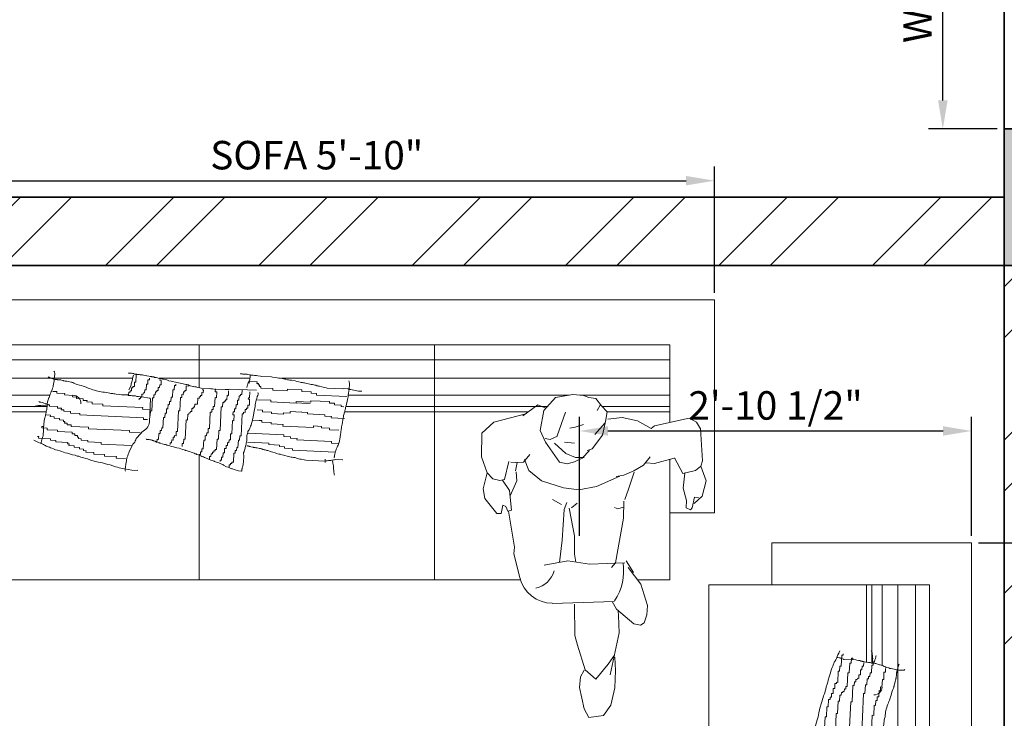
# Model space of a CAD drawing. Units: inches. Extents: x -138 to 270, y 8284 to 8764.
# Tile 8 of 10: x 112 to 198, y 8444 to 8506. Entities that reach past the tile are written whole.
import ezdxf

# ---------------------------------------------------------------- set-up
doc = ezdxf.new("R2010")
doc.units = ezdxf.units.IN
for name, color, linetype, lineweight in [('A-ANNO-DIMS', 2, 'Continuous', 18), ('FURNITURE', 8, 'Continuous', 15), ('FURNITURE1', 8, 'Continuous', 15), ('WALL', 8, 'Continuous', 35)]:
    doc.layers.add(name, color=color, linetype=linetype, lineweight=lineweight)
doc.layers.add('A-COLS', color=252, linetype='Continuous', lineweight=35, true_color=0x939598)
doc.layers.add('A-WALL-PATT', color=32, linetype='Continuous', lineweight=9, true_color=0xbc761a)
doc.styles.get("Standard").update_dxf_attribs({"font": 'arial.ttf'})
doc.dimstyles.new('ISO-25', dxfattribs={"dimtxt": 2.5, "dimasz": 2.5, "dimexe": 1.25, "dimexo": 0.625, "dimtad": 1, "dimdec": 0, "dimlunit": 3, "dimtxsty": 'Standard', "dimcen": 2.5, "dimadec": 0, "dimazin": 0, "dimtfac": 1, "dimtdec": 0, "dimtmove": 0, "dimatfit": 3, "dimfxl": 1, "dimarcsym": 0})

# ---------------------------------------------------------------- blocks, each defined once
blk = doc.blocks.new('A$C48A43CE3')
at = {"layer": 'FURNITURE1', "ltscale": 2}
for p, q in [((21.39, 35.19), (21.36, 35.19)), ((21.42, 35.15), (21.39, 35.19)), ((21.68, 35.14), (21.42, 35.15)), ((21.74, 34.36), (21.64, 34.07)), ((21.77, 35.11), (21.68, 35.14)), ((21.77, 34.49), (21.74, 34.36)), ((21.88, 35.1), (21.77, 35.11)), ((21.78, 34.59), (21.77, 34.49)), ((21.84, 34.84), (21.78, 34.59)), ((21.88, 34.94), (21.84, 34.84)), ((22, 35.06), (21.88, 35.1)), ((21.99, 34.24), (21.97, 33.79)), ((22.13, 34.23), (21.99, 34.24)), ((22.18, 35.06), (22, 35.06)), ((22.16, 34.99), (22.13, 34.23)), ((22.23, 35.02), (22.18, 35.06)), ((22.49, 35.01), (22.23, 35.02)), ((22.58, 34.98), (22.49, 35.01)), ((22.79, 34.97), (22.58, 34.98)), ((22.9, 34.93), (22.79, 34.97)), ((23.08, 34.92), (22.9, 34.93)), ((23.25, 34.88), (23.08, 34.92)), ((23.45, 34.84), (23.25, 34.88)), ((23.36, 34.48), (23.34, 34.03)), ((23.5, 34.47), (23.36, 34.48)), ((23.6, 34.81), (23.45, 34.84)), ((23.5, 34.62), (23.5, 34.47)), ((23.71, 34.8), (23.6, 34.81)), ((23.77, 34.77), (23.71, 34.8)), ((23.95, 34.76), (23.77, 34.77)), ((24.03, 34.72), (23.95, 34.76)), ((24.18, 34.72), (24.03, 34.72)), ((24.32, 34.68), (24.18, 34.72)), ((24.41, 34.64), (24.32, 34.68)), ((24.52, 34.61), (24.41, 34.64)), ((24.64, 34.6), (24.52, 34.61)), ((24.59, 34.57), (24.58, 34.42)), ((24.58, 34.42), (24.72, 34.41)), ((24.73, 34.57), (24.64, 34.6)), ((24.72, 34.41), (24.69, 33.96)), ((24.84, 34.53), (24.73, 34.57)), ((24.96, 34.52), (24.84, 34.53)), ((25.1, 34.49), (24.96, 34.52)), ((25.28, 34.45), (25.1, 34.49)), ((25.48, 34.37), (25.28, 34.45)), ((25.71, 34.33), (25.48, 34.37)), ((26.32, 34.21), (25.71, 34.33)), ((26.49, 34.17), (26.32, 34.21)), ((26.64, 34.13), (26.49, 34.17)), ((33.66, 34.31), (33.53, 34.06)), ((33.67, 34.14), (33.53, 34.15)), ((33.72, 34.37), (33.66, 34.31)), ((33.68, 34.29), (33.67, 34.14)), ((34.49, 34.25), (33.68, 34.29)), ((33.75, 34.44), (33.72, 34.37)), ((33.74, 35.02), (33.77, 34.92)), ((33.77, 34.92), (33.75, 34.44)), ((34.48, 34.1), (34.49, 34.25)), ((14.06, 33.26), (13.66, 33.27)), ((14.06, 33.1), (14.06, 33.26)), ((21.4, 33.21), (21.38, 32.91)), ((21.53, 33.2), (21.4, 33.21)), ((21.57, 33.75), (21.41, 33.43)), ((21.54, 33.36), (21.53, 33.2)), ((21.68, 33.35), (21.54, 33.36)), ((21.63, 33.94), (21.57, 33.75)), ((21.64, 34.07), (21.63, 33.94)), ((21.69, 33.65), (21.68, 33.35)), ((21.83, 33.64), (21.69, 33.65)), ((21.83, 33.79), (21.83, 33.64)), ((21.97, 33.79), (21.83, 33.79)), ((22.89, 33.14), (22.88, 32.99)), ((23.02, 33.13), (22.89, 33.14)), ((23.04, 33.44), (23.02, 33.13)), ((23.17, 33.43), (23.04, 33.44)), ((23.2, 34.03), (23.17, 33.43)), ((23.34, 34.03), (23.2, 34.03)), ((24.12, 33.23), (24.1, 32.93)), ((24.25, 33.23), (24.12, 33.23)), ((24.26, 33.38), (24.25, 33.23)), ((24.39, 33.37), (24.26, 33.38)), ((24.41, 33.67), (24.39, 33.37)), ((24.54, 33.67), (24.41, 33.67)), ((24.56, 33.97), (24.54, 33.67)), ((24.69, 33.96), (24.56, 33.97)), ((25.89, 33.45), (25.86, 32.7)), ((26.03, 33.45), (25.89, 33.45)), ((26.05, 33.9), (26.03, 33.45)), ((26.19, 33.89), (26.05, 33.9)), ((26.19, 34.04), (26.19, 33.89)), ((26.81, 34.09), (26.64, 34.13)), ((27.1, 34.02), (26.81, 34.09)), ((26.97, 33.25), (26.96, 32.95)), ((27.11, 33.24), (26.97, 33.25)), ((27.21, 33.98), (27.1, 34.02)), ((27.11, 33.39), (27.11, 33.24)), ((27.25, 33.39), (27.11, 33.39)), ((27.33, 33.98), (27.21, 33.98)), ((27.27, 33.84), (27.25, 33.39)), ((27.54, 33.83), (27.27, 33.84)), ((27.42, 33.94), (27.33, 33.98)), ((27.48, 33.94), (27.42, 33.94)), ((27.56, 33.9), (27.48, 33.94)), ((27.62, 33.87), (27.56, 33.9)), ((27.71, 33.86), (27.62, 33.87)), ((27.94, 33.79), (27.71, 33.86)), ((28.02, 33.79), (27.94, 33.79)), ((28.14, 33.75), (28.02, 33.79)), ((28.26, 33.75), (28.14, 33.75)), ((28.34, 33.71), (28.26, 33.75)), ((28.46, 33.67), (28.34, 33.71)), ((28.66, 33.66), (28.46, 33.67)), ((28.78, 33.63), (28.66, 33.66)), ((29.62, 33.59), (28.78, 33.63)), ((28.87, 33.16), (28.85, 32.86)), ((29, 33.15), (28.87, 33.16)), ((28.88, 33.46), (29.02, 33.46)), ((29.02, 33.46), (29, 33.15)), ((29.77, 33.56), (29.62, 33.59)), ((29.94, 33.55), (29.77, 33.56)), ((30.12, 33.51), (29.94, 33.55)), ((31.23, 33.47), (30.12, 33.51)), ((30.24, 33.55), (30.23, 33.25)), ((30.23, 33.25), (30.37, 33.24)), ((30.37, 33.24), (30.34, 32.64)), ((31.34, 33.49), (31.23, 33.47)), ((31.61, 33.48), (31.34, 33.49)), ((31.59, 33.33), (31.57, 32.88)), ((31.72, 33.51), (31.61, 33.48)), ((34.44, 33.4), (31.72, 33.51)), ((32.96, 33.42), (32.93, 32.97)), ((33.46, 33.73), (33.45, 33.67)), ((33.49, 33.77), (33.46, 33.73)), ((33.52, 33.93), (33.49, 33.86)), ((33.49, 33.86), (33.49, 33.77)), ((33.53, 34.06), (33.52, 33.93)), ((33.76, 33.23), (33.73, 32.63)), ((34.62, 34.1), (34.48, 34.1)), ((34.57, 33.17), (34.6, 33.1)), ((34.61, 33.95), (34.62, 34.1)), ((34.75, 33.94), (34.61, 33.95)), ((34.74, 33.79), (34.75, 33.94)), ((34.88, 33.78), (34.74, 33.79)), ((34.87, 33.63), (34.88, 33.78)), ((36.09, 33.57), (34.87, 33.63)), ((36.08, 33.42), (36.09, 33.57)), ((37.57, 33.35), (36.08, 33.42)), ((37.58, 33.5), (37.57, 33.35)), ((39.07, 33.43), (37.58, 33.5)), ((39.06, 33.28), (39.07, 33.43)), ((40.01, 33.24), (39.06, 33.28)), ((40.01, 33.09), (40.01, 33.24)), ((12.33, 32.2), (12.24, 32.24)), ((12.45, 32.2), (12.33, 32.2)), ((12.59, 32.16), (12.45, 32.2)), ((12.73, 32.09), (12.59, 32.16)), ((14.87, 33.07), (14.06, 33.1)), ((14.86, 32.92), (14.87, 33.07)), ((15.68, 32.88), (14.86, 32.92)), ((15.67, 32.73), (15.68, 32.88)), ((16.08, 32.71), (15.67, 32.73)), ((16.07, 32.56), (16.08, 32.71)), ((16.75, 32.53), (16.07, 32.56)), ((16.74, 32.37), (16.75, 32.53)), ((17.15, 32.36), (16.74, 32.37)), ((17.14, 32.21), (17.15, 32.36)), ((17.68, 32.18), (17.14, 32.21)), ((17.67, 32.03), (17.68, 32.18)), ((22.45, 32.56), (22.45, 32.41)), ((22.59, 32.55), (22.45, 32.56)), ((22.6, 32.7), (22.59, 32.55)), ((22.73, 32.7), (22.6, 32.7)), ((22.75, 33), (22.73, 32.7)), ((22.88, 32.99), (22.75, 33)), ((23.62, 32.57), (23.52, 30.17)), ((23.82, 32.64), (23.75, 31.29)), ((23.95, 32.64), (23.82, 32.64)), ((23.97, 32.94), (23.95, 32.64)), ((24.1, 32.93), (23.97, 32.94)), ((25.56, 32.26), (25.55, 31.96)), ((25.7, 32.25), (25.56, 32.26)), ((25.72, 32.71), (25.7, 32.25)), ((25.86, 32.7), (25.72, 32.71)), ((26.67, 32.66), (26.61, 31.31)), ((26.81, 32.65), (26.67, 32.66)), ((26.82, 32.96), (26.81, 32.65)), ((26.96, 32.95), (26.82, 32.96)), ((28.43, 32.58), (28.4, 31.98)), ((28.57, 32.57), (28.43, 32.58)), ((28.58, 32.72), (28.57, 32.57)), ((28.71, 32.72), (28.58, 32.72)), ((28.72, 32.87), (28.71, 32.72)), ((28.85, 32.86), (28.72, 32.87)), ((30.2, 32.65), (30.16, 31.74)), ((30.34, 32.64), (30.2, 32.65)), ((30.99, 32.16), (30.97, 31.7)), ((31.13, 32.15), (30.99, 32.16)), ((31.14, 32.3), (31.13, 32.15)), ((31.27, 32.29), (31.14, 32.3)), ((31.28, 32.44), (31.27, 32.29)), ((31.42, 32.44), (31.28, 32.44)), ((31.44, 32.89), (31.42, 32.44)), ((31.57, 32.88), (31.44, 32.89)), ((32.5, 32.39), (32.48, 31.93)), ((32.64, 32.38), (32.5, 32.39)), ((32.66, 32.83), (32.64, 32.38)), ((32.79, 32.82), (32.66, 32.83)), ((32.8, 32.98), (32.79, 32.82)), ((32.93, 32.97), (32.8, 32.98)), ((33.6, 32.64), (33.59, 32.49)), ((33.59, 32.49), (33.73, 32.48)), ((33.73, 32.63), (33.6, 32.64)), ((33.73, 32.48), (33.7, 31.88)), ((34.4, 32.4), (34.29, 31.92)), ((34.46, 32.56), (34.4, 32.4)), ((34.5, 32.75), (34.46, 32.56)), ((34.56, 32.88), (34.5, 32.75)), ((35.9, 32.38), (34.54, 32.44)), ((34.6, 33.01), (34.56, 32.88)), ((34.6, 33.1), (34.6, 33.01)), ((35.89, 32.23), (35.9, 32.38)), ((38.46, 32.1), (35.89, 32.23)), ((38.47, 32.26), (38.46, 32.1)), ((39.96, 32.18), (38.47, 32.26)), ((39.97, 32.34), (39.96, 32.18)), ((41.87, 32.25), (39.97, 32.34)), ((40.55, 33.06), (40.01, 33.09)), ((40.54, 32.91), (40.55, 33.06)), ((43.66, 32.76), (40.54, 32.91)), ((41.86, 32.1), (41.87, 32.25)), ((11.81, 31.73), (11.75, 31.7)), ((11.9, 31.76), (11.81, 31.73)), ((11.93, 31.8), (11.9, 31.76)), ((11.99, 31.79), (11.93, 31.8)), ((12.02, 31.82), (11.99, 31.79)), ((12.14, 31.82), (12.02, 31.82)), ((12.2, 31.85), (12.14, 31.82)), ((12.43, 31.84), (12.2, 31.85)), ((12.58, 31.87), (12.43, 31.84)), ((12.72, 31.86), (12.58, 31.87)), ((12.87, 31.89), (12.72, 31.86)), ((12.91, 32.05), (12.73, 32.09)), ((12.99, 31.88), (12.87, 31.89)), ((13.02, 32.01), (12.91, 32.05)), ((13.11, 31.91), (12.99, 31.88)), ((13.25, 31.91), (13.11, 31.91)), ((13.32, 31.93), (13.19, 31.94)), ((13.31, 31.78), (13.32, 31.93)), ((14.13, 31.74), (13.31, 31.78)), ((14.12, 31.59), (14.13, 31.74)), ((14.53, 31.57), (14.12, 31.59)), ((14.52, 31.42), (14.53, 31.57)), ((14.79, 31.41), (14.52, 31.42)), ((14.78, 31.26), (14.79, 31.41)), ((15.46, 31.23), (14.78, 31.26)), ((15.46, 31.08), (15.46, 31.23)), ((18.76, 31.98), (17.67, 32.03)), ((18.75, 31.83), (18.76, 31.98)), ((22.82, 31.64), (18.75, 31.83)), ((22.81, 31.48), (22.82, 31.64)), ((23.62, 31.45), (22.81, 31.48)), ((23.62, 31.3), (23.6, 30.84)), ((23.75, 31.29), (23.62, 31.3)), ((25.26, 31.52), (25.24, 31.07)), ((25.39, 31.51), (25.26, 31.52)), ((25.42, 31.97), (25.39, 31.51)), ((25.55, 31.96), (25.42, 31.97)), ((26.47, 31.31), (26.37, 29.2)), ((26.61, 31.31), (26.47, 31.31)), ((27.69, 31.25), (27.68, 31.1)), ((27.83, 31.25), (27.69, 31.25)), ((27.84, 31.55), (27.83, 31.25)), ((27.98, 31.54), (27.84, 31.55)), ((27.98, 31.69), (27.98, 31.54)), ((28.12, 31.69), (27.98, 31.69)), ((28.13, 31.99), (28.12, 31.69)), ((28.4, 31.98), (28.13, 31.99)), ((29.72, 31.16), (29.65, 29.5)), ((29.86, 31.15), (29.72, 31.16)), ((29.87, 31.45), (29.86, 31.15)), ((30.01, 31.45), (29.87, 31.45)), ((30.02, 31.75), (30.01, 31.45)), ((30.16, 31.74), (30.02, 31.75)), ((30.84, 31.71), (30.72, 29.3)), ((30.97, 31.7), (30.84, 31.71)), ((32.04, 31.2), (32.02, 30.9)), ((32.17, 31.19), (32.04, 31.2)), ((32.19, 31.5), (32.17, 31.19)), ((32.32, 31.49), (32.19, 31.5)), ((32.34, 31.94), (32.32, 31.49)), ((32.48, 31.93), (32.34, 31.94)), ((33.12, 31.15), (33.11, 31)), ((33.26, 31.14), (33.12, 31.15)), ((33.27, 31.44), (33.26, 31.14)), ((33.41, 31.44), (33.27, 31.44)), ((33.41, 31.59), (33.41, 31.44)), ((33.55, 31.58), (33.41, 31.59)), ((33.56, 31.88), (33.55, 31.58)), ((33.7, 31.88), (33.56, 31.88)), ((34.2, 31.27), (34.13, 30.88)), ((34.21, 31.43), (34.2, 31.27)), ((34.28, 31.75), (34.21, 31.43)), ((34.29, 31.92), (34.28, 31.75)), ((35.03, 31.36), (34.49, 31.39)), ((35.03, 31.21), (35.03, 31.36)), ((35.97, 31.17), (35.03, 31.21)), ((35.97, 31.02), (35.97, 31.17)), ((37.88, 31.23), (37.87, 31.08)), ((39.64, 31.14), (37.88, 31.23)), ((38.2, 32.11), (39.91, 32.05)), ((39.02, 31.23), (39.02, 31.23)), ((39.63, 30.99), (39.64, 31.14)), ((42.4, 32.07), (41.86, 32.1)), ((42.4, 31.92), (42.4, 32.07)), ((43.07, 31.89), (42.4, 31.92)), ((43.07, 31.74), (43.07, 31.89)), ((43.34, 31.72), (43.07, 31.74)), ((13.41, 30.87), (13, 30.89)), ((13.4, 30.72), (13.41, 30.87)), ((13.81, 30.7), (13.4, 30.72)), ((13.8, 30.55), (13.81, 30.7)), ((14.34, 30.53), (13.8, 30.55)), ((14.34, 30.38), (14.34, 30.53)), ((14.74, 30.36), (14.34, 30.38)), ((14.73, 30.21), (14.74, 30.36)), ((14.87, 30.2), (14.73, 30.21)), ((14.86, 30.05), (14.87, 30.2)), ((16.4, 31.03), (15.46, 31.08)), ((16.4, 30.88), (16.4, 31.03)), ((22.9, 30.58), (16.4, 30.88)), ((22.9, 30.42), (22.9, 30.58)), ((23.3, 30.41), (22.9, 30.42)), ((23.52, 30.17), (23.49, 30.01)), ((24.94, 30.63), (24.89, 29.58)), ((25.08, 30.62), (24.94, 30.63)), ((25.1, 31.08), (25.08, 30.62)), ((25.24, 31.07), (25.1, 31.08)), ((27.24, 30.37), (27.15, 28.41)), ((27.38, 30.36), (27.24, 30.37)), ((27.41, 30.97), (27.38, 30.36)), ((27.54, 30.96), (27.41, 30.97)), ((27.55, 31.11), (27.54, 30.96)), ((27.68, 31.1), (27.55, 31.11)), ((31.99, 30.3), (31.93, 28.94)), ((32.13, 30.29), (31.99, 30.3)), ((32.02, 30.9), (32.16, 30.89)), ((32.16, 30.89), (32.13, 30.29)), ((32.98, 31.01), (32.87, 28.75)), ((33.11, 31), (32.98, 31.01)), ((33.98, 30.21), (33.92, 30.02)), ((34.02, 30.43), (33.98, 30.21)), ((34.09, 30.66), (34.02, 30.43)), ((34.85, 30.31), (34.03, 30.35)), ((34.13, 30.88), (34.09, 30.66)), ((34.71, 30.32), (34.85, 30.31)), ((34.98, 30.31), (34.71, 30.32)), ((34.98, 30.16), (34.98, 30.31)), ((35.92, 30.11), (34.98, 30.16)), ((37.19, 30.96), (35.97, 31.02)), ((37.19, 31.11), (37.19, 30.96)), ((37.87, 31.08), (37.19, 31.11)), ((41.4, 30.91), (39.63, 30.99)), ((41.39, 30.76), (41.4, 30.91)), ((42.07, 30.73), (41.39, 30.76)), ((42.06, 30.58), (42.07, 30.73)), ((43.42, 30.51), (42.06, 30.58)), ((12.53, 29.56), (12.54, 29.71)), ((13.07, 29.53), (12.53, 29.56)), ((12.54, 29.71), (12.67, 29.7)), ((13.07, 29.38), (13.07, 29.53)), ((14.15, 29.33), (13.07, 29.38)), ((14.14, 29.18), (14.15, 29.33)), ((15.63, 29.11), (14.14, 29.18)), ((15.13, 30.04), (14.86, 30.05)), ((15.13, 29.89), (15.13, 30.04)), ((15.53, 29.87), (15.13, 29.89)), ((15.53, 29.72), (15.53, 29.87)), ((17.29, 29.63), (15.53, 29.72)), ((17.28, 29.48), (17.29, 29.63)), ((21.48, 29.28), (17.28, 29.48)), ((21.48, 29.13), (21.48, 29.28)), ((22.56, 29.08), (21.48, 29.13)), ((22.75, 29.13), (22.66, 29.03)), ((22.87, 29.22), (22.75, 29.13)), ((22.99, 29.34), (22.87, 29.22)), ((23.14, 29.44), (22.99, 29.34)), ((23.23, 29.53), (23.14, 29.44)), ((23.33, 29.66), (23.23, 29.53)), ((23.39, 29.75), (23.33, 29.66)), ((23.45, 29.88), (23.39, 29.75)), ((23.49, 30.01), (23.45, 29.88)), ((24.61, 29.29), (24.6, 28.99)), ((24.75, 29.28), (24.61, 29.29)), ((24.76, 29.58), (24.75, 29.28)), ((24.89, 29.58), (24.76, 29.58)), ((26.24, 29.21), (26.22, 28.76)), ((26.37, 29.2), (26.24, 29.21)), ((29.51, 29.51), (29.49, 29.06)), ((29.65, 29.5), (29.51, 29.51)), ((30.59, 29.31), (30.55, 28.4)), ((30.72, 29.3), (30.59, 29.31)), ((33.56, 29.19), (33.53, 29.09)), ((33.63, 29.31), (33.56, 29.19)), ((33.69, 29.38), (33.63, 29.31)), ((33.72, 29.44), (33.69, 29.38)), ((33.75, 29.53), (33.72, 29.44)), ((33.78, 29.6), (33.75, 29.53)), ((33.82, 29.73), (33.78, 29.6)), ((33.88, 29.85), (33.82, 29.73)), ((33.92, 30.02), (33.88, 29.85)), ((35.92, 29.96), (35.92, 30.11)), ((37.14, 29.9), (35.92, 29.96)), ((37.13, 29.75), (37.14, 29.9)), ((40.25, 29.61), (37.13, 29.75)), ((40.26, 29.76), (40.25, 29.61)), ((41.07, 29.72), (40.26, 29.76)), ((41.06, 29.57), (41.07, 29.72)), ((41.88, 29.53), (41.06, 29.57)), ((41.87, 29.38), (41.88, 29.53)), ((42.82, 29.33), (41.87, 29.38)), ((12.08, 28.67), (12.22, 28.67)), ((12.22, 28.67), (12.08, 28.67)), ((12.21, 28.51), (12.22, 28.67)), ((13.43, 28.46), (12.21, 28.51)), ((13.42, 28.31), (13.43, 28.46)), ((13.96, 28.28), (13.42, 28.31)), ((13.96, 28.13), (13.96, 28.28)), ((15.18, 28.07), (13.96, 28.13)), ((15.63, 28.96), (15.63, 29.11)), ((15.9, 28.94), (15.63, 28.96)), ((15.89, 28.79), (15.9, 28.94)), ((16.16, 28.78), (15.89, 28.79)), ((16.16, 28.63), (16.16, 28.78)), ((16.29, 28.62), (16.16, 28.63)), ((16.28, 28.47), (16.29, 28.62)), ((16.55, 28.46), (16.28, 28.47)), ((16.55, 28.31), (16.55, 28.46)), ((17.23, 28.28), (16.55, 28.31)), ((17.22, 28.13), (17.23, 28.28)), ((18.57, 28.06), (17.22, 28.13)), ((22.07, 28.24), (22.01, 28.12)), ((22.13, 28.34), (22.07, 28.24)), ((22.17, 28.47), (22.13, 28.34)), ((22.23, 28.56), (22.17, 28.47)), ((22.57, 28.91), (22.23, 28.56)), ((22.66, 29.03), (22.57, 28.91)), ((23.22, 28.39), (23.16, 28.43)), ((23.48, 28.38), (23.22, 28.39)), ((23.57, 28.35), (23.48, 28.38)), ((23.68, 28.34), (23.57, 28.35)), ((23.74, 28.31), (23.68, 28.34)), ((23.8, 28.31), (23.74, 28.31)), ((23.82, 28.27), (23.8, 28.31)), ((23.88, 28.27), (23.82, 28.27)), ((23.91, 28.24), (23.88, 28.27)), ((23.97, 28.23), (23.91, 28.24)), ((24.03, 28.2), (23.97, 28.23)), ((24.11, 28.2), (24.03, 28.2)), ((24.14, 28.16), (24.11, 28.2)), ((24.2, 28.16), (24.14, 28.16)), ((24.26, 28.13), (24.2, 28.16)), ((24.34, 28.12), (24.26, 28.13)), ((24.3, 28.4), (24.28, 28.1)), ((24.43, 28.39), (24.3, 28.4)), ((24.46, 28.05), (24.34, 28.12)), ((24.46, 28.99), (24.43, 28.39)), ((24.6, 28.99), (24.46, 28.99)), ((25.79, 28.33), (25.77, 28.03)), ((25.92, 28.32), (25.79, 28.33)), ((25.94, 28.62), (25.92, 28.32)), ((26.07, 28.62), (25.94, 28.62)), ((26.08, 28.77), (26.07, 28.62)), ((26.22, 28.76), (26.08, 28.77)), ((27.01, 28.42), (26.99, 27.97)), ((27.15, 28.41), (27.01, 28.42)), ((29.05, 28.32), (29, 27.42)), ((29.18, 28.32), (29.05, 28.32)), ((29.2, 28.77), (29.18, 28.32)), ((29.34, 28.76), (29.2, 28.77)), ((29.35, 29.06), (29.34, 28.76)), ((29.49, 29.06), (29.35, 29.06)), ((30.41, 28.41), (30.36, 27.36)), ((30.55, 28.4), (30.41, 28.41)), ((31.63, 28.35), (31.62, 28.05)), ((31.77, 28.35), (31.63, 28.35)), ((31.79, 28.95), (31.77, 28.35)), ((31.93, 28.94), (31.79, 28.95)), ((32.58, 28.31), (32.54, 27.56)), ((32.71, 28.3), (32.58, 28.31)), ((32.74, 28.75), (32.71, 28.3)), ((32.87, 28.75), (32.74, 28.75)), ((33.4, 28.19), (33.39, 27.96)), ((33.44, 28.25), (33.4, 28.19)), ((33.46, 28.8), (33.44, 28.25)), ((33.52, 28.99), (33.46, 28.8)), ((33.53, 29.09), (33.52, 28.99)), ((37.22, 28.84), (33.56, 29.02)), ((37.22, 28.69), (37.22, 28.84)), ((37.89, 28.66), (37.22, 28.69)), ((37.89, 28.51), (37.89, 28.66)), ((38.57, 28.48), (37.89, 28.51)), ((38.56, 28.33), (38.57, 28.48)), ((42.08, 28.16), (38.56, 28.33)), ((42.08, 28.01), (42.08, 28.16)), ((15.17, 27.92), (15.18, 28.07)), ((15.31, 27.92), (15.17, 27.92)), ((15.3, 27.77), (15.31, 27.92)), ((15.84, 27.74), (15.3, 27.77)), ((15.83, 27.59), (15.84, 27.74)), ((16.38, 27.56), (15.83, 27.59)), ((16.37, 27.41), (16.38, 27.56)), ((16.78, 27.39), (16.37, 27.41)), ((16.77, 27.24), (16.78, 27.39)), ((17.04, 27.23), (16.77, 27.24)), ((17.03, 27.08), (17.04, 27.23)), ((18.57, 27.91), (18.57, 28.06)), ((21.68, 27.77), (18.57, 27.91)), ((21.44, 27.13), (21.41, 27.01)), ((21.51, 27.29), (21.44, 27.13)), ((21.7, 27.68), (21.51, 27.29)), ((21.76, 27.77), (21.7, 27.68)), ((21.82, 27.9), (21.76, 27.77)), ((21.92, 28.02), (21.82, 27.9)), ((22.01, 28.12), (21.92, 28.02)), ((24.28, 28.1), (24.15, 28.1)), ((24.52, 28.05), (24.46, 28.05)), ((24.57, 28.02), (24.52, 28.05)), ((24.63, 28.01), (24.57, 28.02)), ((24.8, 27.94), (24.63, 28.01)), ((25.04, 27.87), (24.8, 27.94)), ((25.15, 27.86), (25.04, 27.87)), ((25.24, 27.83), (25.15, 27.86)), ((25.3, 27.79), (25.24, 27.83)), ((25.35, 27.79), (25.3, 27.79)), ((25.44, 27.75), (25.35, 27.79)), ((25.58, 27.72), (25.44, 27.75)), ((25.76, 27.68), (25.58, 27.72)), ((25.64, 28.03), (25.63, 27.88)), ((25.77, 28.03), (25.64, 28.03)), ((25.96, 27.64), (25.76, 27.68)), ((26.31, 27.53), (25.96, 27.64)), ((26.54, 27.48), (26.31, 27.53)), ((26.88, 27.37), (26.54, 27.48)), ((26.86, 27.97), (26.84, 27.67)), ((26.99, 27.97), (26.86, 27.97)), ((27.06, 27.33), (26.88, 27.37)), ((27.14, 27.3), (27.06, 27.33)), ((27.2, 27.26), (27.14, 27.3)), ((27.26, 27.26), (27.2, 27.26)), ((27.35, 27.22), (27.26, 27.26)), ((27.46, 27.19), (27.35, 27.22)), ((27.61, 27.15), (27.46, 27.19)), ((27.75, 27.08), (27.61, 27.15)), ((28.72, 27.13), (28.71, 26.83)), ((28.86, 27.13), (28.72, 27.13)), ((28.87, 27.43), (28.86, 27.13)), ((29, 27.42), (28.87, 27.43)), ((30.08, 27.22), (30.08, 27.07)), ((30.22, 27.21), (30.08, 27.22)), ((30.23, 27.36), (30.22, 27.21)), ((30.36, 27.36), (30.23, 27.36)), ((31.18, 27.47), (31.16, 27.02)), ((31.32, 27.46), (31.18, 27.47)), ((31.33, 27.76), (31.32, 27.46)), ((31.47, 27.76), (31.33, 27.76)), ((31.48, 28.06), (31.47, 27.76)), ((31.62, 28.05), (31.48, 28.06)), ((32.26, 27.27), (32.24, 26.97)), ((32.39, 27.26), (32.26, 27.27)), ((32.41, 27.56), (32.39, 27.26)), ((32.54, 27.56), (32.41, 27.56)), ((33.16, 27.12), (33.12, 27.06)), ((33.26, 27.48), (33.16, 27.19)), ((33.16, 27.19), (33.16, 27.12)), ((33.3, 27.67), (33.26, 27.57)), ((33.26, 27.57), (33.26, 27.48)), ((33.36, 27.86), (33.3, 27.74)), ((33.3, 27.74), (33.3, 27.67)), ((33.39, 27.96), (33.36, 27.93)), ((33.36, 27.93), (33.36, 27.86)), ((35.69, 28.01), (33.52, 28.11)), ((35.68, 27.86), (35.69, 28.01)), ((36.77, 27.81), (35.68, 27.86)), ((36.76, 27.66), (36.77, 27.81)), ((37.3, 27.63), (36.76, 27.66)), ((37.3, 27.48), (37.3, 27.63)), ((38.11, 27.44), (37.3, 27.48)), ((38.1, 27.29), (38.11, 27.44)), ((42.44, 27.09), (38.1, 27.29)), ((42.75, 27.98), (42.08, 28.01)), ((17.85, 27.04), (17.03, 27.08)), ((17.84, 26.89), (17.85, 27.04)), ((18.92, 26.84), (17.84, 26.89)), ((18.92, 26.69), (18.92, 26.84)), ((20.14, 26.63), (18.92, 26.69)), ((20.13, 26.48), (20.14, 26.63)), ((21.08, 26.44), (20.13, 26.48)), ((21.17, 26.17), (21.13, 26.07)), ((21.21, 26.46), (21.17, 26.3)), ((21.17, 26.3), (21.17, 26.17)), ((21.24, 26.59), (21.21, 26.46)), ((21.31, 26.72), (21.24, 26.59)), ((21.34, 26.88), (21.31, 26.72)), ((21.41, 27.01), (21.34, 26.88)), ((27.98, 27), (27.75, 27.08)), ((28.07, 26.97), (27.98, 27)), ((28.12, 26.97), (28.07, 26.97)), ((28.15, 26.93), (28.12, 26.97)), ((28.21, 26.93), (28.15, 26.93)), ((28.27, 26.9), (28.21, 26.93)), ((28.35, 26.86), (28.27, 26.9)), ((28.5, 26.82), (28.35, 26.86)), ((28.61, 26.78), (28.5, 26.82)), ((28.71, 26.83), (28.57, 26.84)), ((28.76, 26.71), (28.61, 26.78)), ((28.87, 26.64), (28.76, 26.71)), ((28.96, 26.61), (28.87, 26.64)), ((29.02, 26.61), (28.96, 26.61)), ((29.13, 26.54), (29.02, 26.61)), ((29.24, 26.5), (29.13, 26.54)), ((29.76, 26.28), (29.24, 26.5)), ((29.65, 26.64), (29.63, 26.34)), ((29.78, 26.63), (29.65, 26.64)), ((29.91, 26.25), (29.76, 26.28)), ((29.8, 26.93), (29.78, 26.63)), ((29.93, 26.92), (29.8, 26.93)), ((30.02, 26.21), (29.91, 26.25)), ((29.94, 27.07), (29.93, 26.92)), ((30.08, 27.07), (29.94, 27.07)), ((30.11, 26.17), (30.02, 26.21)), ((30.16, 26.14), (30.11, 26.17)), ((30.25, 26.1), (30.16, 26.14)), ((30.72, 26.28), (30.71, 26.13)), ((30.85, 26.28), (30.72, 26.28)), ((30.87, 26.58), (30.85, 26.28)), ((31, 26.57), (30.87, 26.58)), ((31.02, 27.02), (31, 26.57)), ((31.16, 27.02), (31.02, 27.02)), ((32.11, 26.97), (32.07, 26.07)), ((32.24, 26.97), (32.11, 26.97)), ((33.12, 27), (33.09, 26.96)), ((33.09, 26.96), (33.09, 26.83)), ((33.09, 26.83), (33.14, 26.77)), ((33.14, 26.77), (33.11, 26.02)), ((33.12, 27.06), (33.12, 27)), ((41.44, 26.02), (41.45, 26.37)), ((42.17, 26.18), (42.23, 26.05)), ((21.06, 25.69), (21.04, 25.23)), ((21.04, 25.23), (21.07, 25.14)), ((21.09, 25.75), (21.06, 25.69)), ((21.1, 25.91), (21.09, 25.75)), ((21.13, 25.98), (21.1, 25.91)), ((21.13, 26.07), (21.13, 25.98)), ((30.6, 25.99), (30.25, 26.1)), ((30.71, 25.92), (30.6, 25.99)), ((30.8, 25.89), (30.71, 25.92)), ((30.91, 25.85), (30.8, 25.89)), ((31, 25.81), (30.91, 25.85)), ((31.08, 25.75), (31, 25.81)), ((31.37, 25.6), (31.08, 25.75)), ((31.54, 25.56), (31.37, 25.6)), ((31.66, 25.5), (31.54, 25.56)), ((31.65, 25.79), (31.63, 25.49)), ((31.78, 25.78), (31.65, 25.79)), ((31.92, 25.39), (31.66, 25.5)), ((31.79, 25.93), (31.78, 25.78)), ((31.92, 25.93), (31.79, 25.93)), ((31.93, 26.08), (31.92, 25.93)), ((31.97, 25.39), (31.92, 25.39)), ((32.07, 26.07), (31.93, 26.08)), ((32.15, 25.31), (31.97, 25.39)), ((32.61, 25.17), (32.15, 25.31)), ((32.9, 25.15), (32.61, 25.17)), ((32.93, 25.19), (32.9, 25.15)), ((32.94, 25.35), (32.93, 25.19)), ((32.97, 25.38), (32.94, 25.35)), ((33, 25.54), (32.97, 25.48)), ((32.97, 25.48), (32.97, 25.38)), ((33.01, 25.6), (33, 25.54)), ((33.04, 25.64), (33.01, 25.6)), ((33.07, 25.8), (33.04, 25.7)), ((33.04, 25.7), (33.04, 25.64)), ((33.08, 25.96), (33.07, 25.8)), ((33.11, 26.02), (33.08, 25.96)), ((42.23, 26.05), (42.22, 25.95)), ((42.22, 25.95), (42.27, 25.69)), ((42.27, 25.69), (42.29, 25.53)), ((42.29, 25.53), (42.29, 25.37)), ((42.29, 25.37), (42.31, 25.2)), ((42.31, 25.2), (42.33, 25.1)), ((42.33, 25.1), (42.33, 25.01)), ((42.33, 25.01), (42.36, 24.94)), ((42.36, 24.94), (42.35, 24.81)), ((42.35, 24.81), (42.38, 24.75))]:
    blk.add_line(p, q, dxfattribs=at)
at = {"layer": 'FURNITURE1'}
for p, q in [((63.73, 31.32), (64.91, 32.67)), ((64.91, 32.67), (66.68, 32.96)), ((66.68, 32.96), (67.78, 32.88)), ((67.78, 32.88), (68.31, 32.65)), ((68.31, 32.65), (69.04, 32.56)), ((69.04, 32.56), (69.62, 31.81)), ((61.6, 30.79), (63.12, 31.91)), ((63.12, 31.91), (63.95, 31.58)), ((63.37, 29.3), (63.73, 31.32)), ((65.11, 28.76), (65.94, 31.18)), ((69.47, 31.89), (69.17, 31.35)), ((69.62, 31.81), (70.21, 31.21)), ((70.21, 31.21), (70.04, 30.22)), ((57.41, 29.03), (58.64, 30.16)), ((58.64, 30.16), (61.89, 31)), ((70.04, 30.22), (69.71, 28.81)), ((71.74, 30.63), (70.26, 30.44)), ((73.3, 30.29), (71.74, 30.63)), ((74.67, 29.49), (73.3, 30.29)), ((78.55, 30.57), (75.04, 29.77)), ((79.32, 30.14), (78.55, 30.57)), ((79.72, 29.45), (79.32, 30.14)), ((63.91, 28.1), (63.37, 29.3)), ((66.93, 29.65), (66.38, 29.55)), ((67.79, 29.92), (66.93, 29.65)), ((68.95, 28.88), (69.95, 30.05)), ((75.04, 29.77), (74.67, 29.49)), ((79.92, 26.2), (79.72, 29.45)), ((57.39, 26.62), (57.41, 29.03)), ((64.38, 28.38), (63.87, 28.49)), ((65.13, 28.73), (64.38, 28.38)), ((66.87, 28.02), (65.83, 28.12)), ((69.71, 28.81), (68.66, 27.41)), ((65.34, 26.06), (63.91, 28.1)), ((65.97, 26.96), (64.81, 28.02)), ((68.4, 27.27), (67.64, 26.48)), ((68.66, 27.41), (68.16, 27.24)), ((57.95, 24.98), (57.39, 26.62)), ((60.16, 26.13), (59.71, 24.29)), ((62.32, 26.83), (61.66, 26.07)), ((62.21, 25.2), (61.78, 26.32)), ((66.97, 26.54), (65.97, 26.96)), ((67.64, 26.48), (66.86, 26.1)), ((67.84, 26.53), (66.97, 26.54)), ((74.59, 26.61), (73.91, 25.77)), ((77.02, 26.46), (75.03, 25.92)), ((77.92, 24.92), (77.07, 26.52)), ((79.75, 25.65), (79.92, 26.2)), ((60.84, 26.02), (60.36, 26.06)), ((61.66, 26.07), (60.84, 26.02)), ((61.03, 26.03), (60.86, 25.18)), ((63.49, 24.17), (62.21, 25.2)), ((66.12, 25.9), (65.34, 26.06)), ((66.86, 26.1), (66.12, 25.9)), ((72.91, 25.18), (71.89, 24.73)), ((73.91, 25.77), (72.91, 25.18)), ((75.03, 25.92), (74.16, 26.01)), ((79.2, 25.21), (77.92, 24.92)), ((79.7, 25.63), (79.2, 25.21)), ((80.29, 24.17), (79.75, 25.65)), ((57.54, 23.33), (57.95, 24.98)), ((57.95, 24.98), (58.54, 24.37)), ((58.54, 24.37), (59.25, 24.18)), ((59.25, 24.18), (59.71, 24.29)), ((59.52, 24.23), (60.23, 23.17)), ((60.98, 24.17), (60.29, 22.63)), ((60.9, 25.08), (60.98, 24.17)), ((65.75, 23.44), (63.49, 24.17)), ((71.49, 24.63), (69.1, 23.59)), ((71.89, 24.73), (71.1, 24.59)), ((72.38, 23.32), (72.95, 25.03)), ((78.13, 24.93), (77.95, 23.41)), ((79.9, 22.59), (80.29, 24.17)), ((57.73, 22.35), (57.54, 23.33)), ((60.23, 23.17), (60.45, 21.16)), ((67.32, 23.24), (65.75, 23.44)), ((69.1, 23.59), (67.32, 23.24)), ((72.01, 22.25), (72.38, 23.32)), ((77.95, 23.41), (78.27, 22.14)), ((58.93, 20.81), (57.73, 22.35)), ((64.63, 22.24), (65.53, 21.74)), ((78.27, 22.14), (78.25, 21.41)), ((78.86, 21.4), (79.09, 22.48)), ((79.08, 21.86), (79.9, 22.59)), ((79.09, 22.48), (79.5, 22.45)), ((59.54, 21.67), (59.4, 20.81)), ((59.85, 21.53), (59.54, 21.67)), ((60.06, 21.08), (59.85, 21.53)), ((60.45, 21.16), (60.06, 21.08)), ((65.61, 18.12), (65.8, 21.23)), ((65.8, 21.23), (66.09, 21.96)), ((66.32, 21.37), (66.87, 18.56)), ((66.56, 21.41), (67.13, 21.88)), ((71.27, 21.29), (70.94, 21.43)), ((71.86, 21.46), (71.27, 21.29)), ((71.86, 20.35), (71.89, 22.08)), ((78.25, 21.41), (78.68, 21.2)), ((78.86, 21.4), (78.68, 21.2)), ((59.4, 20.81), (58.93, 20.81)), ((60.12, 21.08), (60.74, 17.4)), ((71.03, 15.78), (71.86, 20.35)), ((65.32, 15.82), (65.61, 18.12)), ((66.87, 18.6), (66.86, 16.67)), ((60.74, 17.4), (60.69, 16.7)), ((60.69, 16.7), (61.28, 14.28)), ((66.86, 16.67), (67.01, 15.86)), ((66.19, 15.98), (63.76, 15.54)), ((68.41, 15.66), (66.19, 15.98)), ((72.01, 15.78), (68.41, 15.66)), ((70.64, 15.3), (71.03, 15.78)), ((71, 15.74), (70.99, 15.79)), ((72.87, 14.79), (72.13, 16.01)), ((73.63, 13.63), (72.35, 15.33)), ((74.3, 11.44), (73.63, 13.63)), ((64.58, 11.65), (70.9, 11.84)), ((66.91, 8.38), (66.88, 11.59)), ((70.71, 11.83), (71.14, 11.05)), ((71.14, 11.05), (72.9, 9.56)), ((74.23, 10.49), (74.3, 11.44)), ((71.36, 10.43), (71.33, 10.9)), ((71.42, 8.64), (71.36, 10.43)), ((73.96, 9.67), (74.23, 10.49)), ((72.9, 9.56), (73.59, 9.44)), ((73.59, 9.44), (73.96, 9.67)), ((66.91, 8.38), (67.17, 7.38)), ((70.49, 4.37), (71.42, 8.64)), ((67.17, 7.38), (67.94, 4.86)), ((70.29, 5.44), (70.93, 6.37)), ((71.03, 4.82), (70.97, 6.18)), ((69.04, 3.92), (70.29, 5.44)), ((67.47, 4.16), (67.39, 3.07)), ((67.85, 4.84), (67.47, 4.16)), ((67.94, 4.86), (69.04, 3.92)), ((70.99, 3.03), (71.03, 4.82)), ((67.39, 3.07), (67.84, 0.9)), ((70.57, 1.26), (70.99, 3.03)), ((69.82, 0.2), (70.57, 1.26)), ((67.84, 0.9), (68.34, 0)), ((68.34, 0), (69.82, 0.2))]:
    blk.add_line(p, q, dxfattribs=at)
for points in [[(76.57, 20.9), (81.14, 20.9), (81.14, 42.62), (0, 42.62), (0, 20.9), (4.57, 20.9)], [(61.35, 14.04), (4.57, 14.04), (4.57, 38.04), (76.57, 38.04), (76.57, 30.12)], [(4.57, 14.04), (4.57, 38.04)], [(28.57, 33.67), (28.57, 38.04)], [(52.57, 14.04), (52.57, 38.04)], [(76.57, 36.51), (4.57, 36.51)], [(21.78, 34.62), (4.57, 34.62)], [(33.76, 34.62), (24.5, 34.62)], [(76.57, 34.62), (36.97, 34.62)], [(13.35, 32.9), (4.57, 32.9)], [(66.32, 32.9), (43.79, 32.9)], [(76.57, 32.9), (67.44, 32.9)], [(13.07, 31.76), (4.57, 31.76)], [(12.99, 31.19), (4.57, 31.19)], [(62.14, 31.19), (43.41, 31.19)], [(64.11, 31.76), (43.55, 31.76)], [(63.49, 31.76), (64.11, 31.76)], [(64.11, 31.76), (63.49, 31.76)], [(76.57, 31.76), (69.66, 31.76)], [(76.57, 31.19), (70.21, 31.19)], [(28.57, 14.04), (28.57, 26.8)], [(76.57, 26.34), (76.57, 14.04), (73.31, 14.04)]]:
    blk.add_lwpolyline(points, dxfattribs=at)
at = {"layer": 'FURNITURE1', "ltscale": 2}
for points in [[(13.77, 35.36), (13.83, 35.29), (13.83, 35.23), (13.85, 35.16), (13.83, 34.71), (13.8, 34.51), (13.79, 34.35), (13.68, 33.87), (13.68, 33.74), (13.61, 33.61), (13.55, 33.35), (13.48, 33.26), (13.45, 33.13), (13.38, 33), (13.32, 32.81), (13.28, 32.68), (13.25, 32.62), (13.12, 32.23), (13.12, 32.14), (13.08, 32.01), (13.07, 31.75), (13.03, 31.59), (13.03, 31.43), (12.99, 31.27), (12.99, 31.14), (12.95, 30.98), (12.92, 30.88), (12.91, 30.78), (12.88, 30.72), (12.88, 30.65), (12.85, 30.59), (12.81, 30.49), (12.81, 30.43), (12.78, 30.33), (12.77, 30.14), (12.74, 30.04), (12.68, 28.75), (12.65, 28.68), (12.62, 28.59), (12.56, 28.46), (12.55, 28.39), (12.52, 28.33), (12.49, 28.23), (12.48, 28.04), (12.45, 28.01)], [(23.59, 32.6), (23.48, 32.6), (23.3, 32.64), (22.95, 32.69), (22.72, 32.73), (22.4, 32.78), (22.23, 32.78), (22.08, 32.82), (21.76, 32.83), (21.65, 32.87), (21.38, 32.88), (21.27, 32.92), (20.66, 32.94), (20.48, 32.98), (20.13, 33), (19.99, 33.03), (19.87, 33.04), (19.76, 33.08), (19.58, 33.08), (19.47, 33.12), (19.29, 33.13), (19.12, 33.17), (18.91, 33.21), (18.74, 33.21), (18.57, 33.25), (18.42, 33.26), (18.25, 33.3), (18.1, 33.34), (17.9, 33.41), (17.73, 33.45), (17.55, 33.52), (17.41, 33.59), (17.27, 33.63), (17.12, 33.7), (16.89, 33.77), (16.75, 33.81), (16.58, 33.88), (16.37, 33.92), (16.14, 34), (15.94, 34.07), (15.8, 34.14), (15.68, 34.18), (15.62, 34.18), (15.57, 34.22), (15.48, 34.22), (15.25, 34.29), (15.08, 34.33), (14.93, 34.34), (14.81, 34.38), (14.76, 34.38), (14.7, 34.41), (14.55, 34.42), (14.47, 34.45), (14.15, 34.47), (14.09, 34.5), (13.91, 34.51), (13.83, 34.54), (13.74, 34.55), (13.39, 34.66), (13.28, 34.73), (13.22, 34.73), (13.19, 34.76)], [(45.18, 33.3), (44.83, 33.32), (44.37, 33.4), (44.2, 33.44), (44.05, 33.48), (43.96, 33.48), (43.91, 33.51), (43.82, 33.52), (43.79, 33.55), (43.3, 33.57), (43.21, 33.54), (41.63, 33.6), (41.52, 33.64), (41.08, 33.76), (40.85, 33.83), (40.76, 33.83), (40.68, 33.87), (40.59, 33.87), (40.48, 33.91), (40.39, 33.91), (40.27, 33.95), (40.13, 33.99), (40.01, 33.99), (39.72, 34.07), (39.58, 34.08), (39.43, 34.11), (39.32, 34.15), (39.23, 34.15), (39.11, 34.19), (39, 34.2), (38.88, 34.23), (38.74, 34.27), (38.56, 34.31), (38.36, 34.35), (38.01, 34.43), (37.84, 34.44), (37.69, 34.47), (37.58, 34.48), (37.43, 34.52), (37.32, 34.52), (37.2, 34.56), (37.06, 34.6), (36.88, 34.64), (36.71, 34.64), (36.36, 34.72), (36.07, 34.73), (35.95, 34.77), (34.99, 34.81), (34.85, 34.85), (34.55, 34.86), (34.44, 34.9), (34.21, 34.91), (34.09, 34.94), (33.83, 34.95), (33.74, 34.99), (33.54, 35), (33.48, 35.03), (33.04, 35.05), (32.96, 35.08), (32.84, 35.09), (32.81, 35.12)], [(43.85, 34.36), (43.88, 34.29), (43.88, 34.23), (43.9, 34.1), (43.88, 33.48), (43.84, 33.35), (43.83, 33.06), (43.79, 32.9), (43.79, 32.74), (43.75, 32.58), (43.72, 32.45), (43.57, 31.81), (43.51, 31.68), (43.5, 31.55), (43.47, 31.42), (43.44, 31.33), (43.43, 31.23), (43.4, 31.16), (43.37, 31.07), (43.37, 31), (43.3, 30.81), (43.29, 30.68), (43.26, 30.55), (43.22, 30.39), (43.21, 30.1), (43.18, 29.94), (43.11, 29.68), (43.1, 29.55), (43.07, 29.43), (43.06, 29.33), (43.03, 29.2), (43.02, 29.01), (42.99, 28.94), (42.97, 28.59), (42.94, 28.49), (42.94, 28.39), (42.9, 28.3), (42.9, 28.2), (42.77, 27.81), (42.7, 27.69), (42.67, 27.59), (42.57, 27.4), (42.51, 27.21), (42.48, 27.14), (42.44, 27.05), (42.44, 26.98), (42.41, 26.92), (42.4, 26.76), (42.37, 26.73), (42.37, 26.6), (42.34, 26.57), (42.33, 26.53)], [(22.27, 25.25), (22.3, 25.22), (21.71, 25.24), (21.34, 25.32), (20.96, 25.37), (20.76, 25.41), (20.41, 25.49), (20.24, 25.56), (20.06, 25.6), (19.49, 25.78), (19.25, 25.82), (18.91, 25.94), (18.71, 25.98), (18.47, 26.02), (18.16, 26.1), (17.98, 26.13), (17.78, 26.21), (17.61, 26.25), (17.2, 26.39), (17, 26.43), (16.83, 26.5), (16.65, 26.54), (16.51, 26.58), (16.31, 26.66), (16.13, 26.69), (15.93, 26.77), (15.67, 26.81), (15.36, 26.92), (15.15, 26.99), (14.92, 27.03), (14.58, 27.15), (14.37, 27.22), (14.14, 27.29), (13.94, 27.33), (13.74, 27.41), (13.57, 27.48), (13.42, 27.52), (13.31, 27.59), (13.19, 27.62), (13.11, 27.66), (12.99, 27.7), (12.91, 27.76), (12.82, 27.8), (12.71, 27.87), (12.56, 27.94), (12.36, 28.01), (12.19, 28.08), (11.99, 28.19), (11.73, 28.3)], [(43.2, 26.34), (43.17, 26.31), (42.47, 26.33), (42.38, 26.3), (42.3, 26.31), (42.21, 26.28), (42.09, 26.28), (42, 26.25), (41.88, 26.23), (41.77, 26.23), (41.65, 26.2), (41.53, 26.21), (41.39, 26.18), (39.46, 26.26), (39.29, 26.3), (39, 26.37), (38.85, 26.38), (38.71, 26.42), (38.59, 26.45), (38.45, 26.49), (38.33, 26.53), (38.19, 26.54), (38.07, 26.57), (37.95, 26.58), (37.84, 26.61), (37.69, 26.65), (37.17, 26.77), (37.06, 26.81), (36.91, 26.85), (36.83, 26.88), (36.71, 26.89), (36.48, 26.96), (36.34, 27), (36.1, 27.07), (35.96, 27.11), (35.87, 27.15), (35.76, 27.18), (35.59, 27.25), (35.47, 27.26), (35.41, 27.29), (35.33, 27.33), (35.21, 27.33), (35.15, 27.37), (35.07, 27.37), (34.98, 27.41), (34.89, 27.41), (34.83, 27.45), (34.72, 27.45), (34.49, 27.53), (34.37, 27.53), (34.28, 27.57), (34.14, 27.57), (34.08, 27.61), (33.85, 27.62), (33.79, 27.65), (33.73, 27.65), (33.68, 27.69), (33.59, 27.69), (33.53, 27.73), (33.44, 27.73)]]:
    blk.add_lwpolyline(points, dxfattribs=at)
blk.add_arc((15.67, 32.04), 0.857, 358, 88, dxfattribs=at)
at = {"layer": 'FURNITURE1'}
for centre, radius, start, end in [((66.53, 14.94), 5.35, 325.7419, 8.9934), ((64.63, 15.1), 3.44, 193.691, 269.2083), ((62.32, 15.69), 2.57, 283.6862, 343.8561)]:
    blk.add_arc(centre, radius, start, end, dxfattribs=at)
blk = doc.blocks.new('COLUMN-9X12IN')
h = blk.add_hatch(color=256)
h.dxf.hatch_style = 1
h.paths.add_polyline_path([(9, 12), (0, 12), (0, 0), (9, 0)])
blk.add_lwpolyline([(0, 0), (9, 0), (9, 12), (0, 12)], close=True)
blk = doc.blocks.new('*D33')
at = {"layer": 'A-ANNO-DIMS', "color": 0, "lineweight": -2, "transparency": 16777216}
for p, q in [((197.451, 8532.243), (191.426, 8532.243)), ((192.676, 8498.743), (192.676, 8529.743)), ((197.451, 8496.243), (191.426, 8496.243))]:
    blk.add_line(p, q, dxfattribs=at)
at = {"layer": 'A-ANNO-DIMS', "color": 0, "transparency": 16777216}
for points in [[(192.259, 8529.743), (193.092, 8529.743), (192.676, 8532.243)], [(192.259, 8498.743), (193.092, 8498.743), (192.676, 8496.243)]]:
    blk.add_solid(points, dxfattribs=at)
at = {"layer": 'Defpoints', "color": 0, "transparency": 16777216}
for p in [(192.676, 8532.243), (198.076, 8532.243), (198.076, 8496.243)]:
    blk.add_point(p, dxfattribs=at)
at = {"layer": 'A-ANNO-DIMS', "color": 0, "transparency": 16777216, "insert": (190.773, 8514.243), "char_height": 2.5, "attachment_point": 5, "rotation": 90}
blk.add_mtext('W1 3\'-0" TYP.', dxfattribs=at)
blk = doc.blocks.new('*D41')
at = {"layer": 'A-ANNO-DIMS', "color": 0, "lineweight": -2, "transparency": 16777216}
for p, q in [((102.748, 8481.839), (102.748, 8492.945)), ((172.622, 8481.839), (172.622, 8492.945)), ((105.248, 8491.695), (170.122, 8491.695))]:
    blk.add_line(p, q, dxfattribs=at)
at = {"layer": 'A-ANNO-DIMS', "color": 0, "transparency": 16777216}
for points in [[(105.248, 8492.112), (105.248, 8491.279), (102.748, 8491.695)], [(170.122, 8492.112), (170.122, 8491.279), (172.622, 8491.695)]]:
    blk.add_solid(points, dxfattribs=at)
at = {"layer": 'Defpoints', "color": 0, "transparency": 16777216}
for p in [(172.622, 8491.695), (102.748, 8481.214), (172.622, 8481.214)]:
    blk.add_point(p, dxfattribs=at)
at = {"layer": 'A-ANNO-DIMS', "color": 0, "transparency": 16777216, "insert": (137.685, 8493.614), "char_height": 2.5, "attachment_point": 5}
blk.add_mtext('SOFA 5\'-10"', dxfattribs=at)
blk = doc.blocks.new('*D43')
at = {"layer": 'A-ANNO-DIMS', "color": 0, "lineweight": -2, "transparency": 16777216}
for p, q in [((195.822, 8459.87), (206.28, 8459.87)), ((205.03, 8457.37), (205.03, 8396.813)), ((195.822, 8394.313), (206.28, 8394.313))]:
    blk.add_line(p, q, dxfattribs=at)
at = {"layer": 'A-ANNO-DIMS', "color": 0, "transparency": 16777216}
for points in [[(204.614, 8457.37), (205.447, 8457.37), (205.03, 8459.87)], [(204.614, 8396.813), (205.447, 8396.813), (205.03, 8394.313)]]:
    blk.add_solid(points, dxfattribs=at)
at = {"layer": 'Defpoints', "color": 0, "transparency": 16777216}
for p in [(195.197, 8459.87), (195.197, 8394.313), (205.03, 8394.313)]:
    blk.add_point(p, dxfattribs=at)
at = {"layer": 'A-ANNO-DIMS', "color": 0, "transparency": 16777216, "insert": (203.112, 8427.092), "char_height": 2.5, "attachment_point": 5, "rotation": 90}
blk.add_mtext('SOFA 5\'-5 1/2"', dxfattribs=at)
blk = doc.blocks.new('*D44')
at = {"layer": 'A-ANNO-DIMS', "color": 0, "lineweight": -2, "transparency": 16777216}
for p, q in [((160.767, 8460.495), (160.767, 8470.953)), ((195.197, 8460.495), (195.197, 8470.953)), ((163.267, 8469.703), (192.697, 8469.703))]:
    blk.add_line(p, q, dxfattribs=at)
at = {"layer": 'A-ANNO-DIMS', "color": 0, "transparency": 16777216}
for points in [[(163.267, 8470.12), (163.267, 8469.287), (160.767, 8469.703)], [(192.697, 8470.12), (192.697, 8469.287), (195.197, 8469.703)]]:
    blk.add_solid(points, dxfattribs=at)
at = {"layer": 'Defpoints', "color": 0, "transparency": 16777216}
for p in [(195.197, 8469.703), (160.767, 8459.87), (195.197, 8459.87)]:
    blk.add_point(p, dxfattribs=at)
at = {"layer": 'A-ANNO-DIMS', "color": 0, "transparency": 16777216, "insert": (177.982, 8471.621), "char_height": 2.5, "attachment_point": 5}
blk.add_mtext('2\'-10 1/2"', dxfattribs=at)

msp = doc.modelspace()

# ---------------------------------------------------------------- hatches: boundary and pattern name
at = {"layer": 'A-WALL-PATT'}
h = msp.add_hatch(dxfattribs=at)
h.set_pattern_fill('ANSI32', color=256)
h.paths.add_polyline_path([(115.814, 8699.243), (65.223, 8699.243), (65.223, 8690.243), (68.076, 8690.243), (68.076, 8686.356), (69.019, 8686.356), (69.019, 8686.356), (73.519, 8686.356), (74.076, 8686.356), (74.076, 8690.243), (115.814, 8690.243)])
h.paths.add_polyline_path([(169.814, 8699.243), (139.814, 8699.243), (139.814, 8690.243), (169.814, 8690.243)])
h.paths.add_polyline_path([(198.076, 8699.243), (193.814, 8699.243), (193.814, 8690.243), (198.076, 8690.243)])
h.paths.add_polyline_path([(207.076, 8648.243), (204.227, 8648.243), (204.227, 8648.243), (199.727, 8648.243), (198.076, 8648.243), (198.076, 8642.243), (150.076, 8642.243), (150.076, 8690.243), (144.076, 8690.243), (144.076, 8642.243), (74.076, 8642.243), (74.076, 8653.356), (68.076, 8653.356), (68.076, 8526.241), (68.826, 8526.241), (74.076, 8526.241), (74.076, 8630.243), (74.076, 8636.243), (98.076, 8636.243), (150.076, 8636.243), (198.076, 8636.243), (198.076, 8630.243), (198.076, 8532.243), (207.076, 8532.243)])
h.paths.add_polyline_path([(207.076, 8484.243), (198.076, 8484.243), (198.076, 8433.433), (207.076, 8433.433)])
h.paths.add_polyline_path([(198.076, 8490.243), (80.076, 8490.243), (80.076, 8484.243), (198.076, 8484.243)])
h.paths.add_polyline_path([(207.076, 8397.433), (198.076, 8397.433), (198.076, 8359.273), (207.076, 8359.273)])
h.paths.add_polyline_path([(198.076, 8356.243), (186.078, 8356.243), (186.078, 8347.243), (198.076, 8347.243)])
h.paths.add_polyline_path([(138.078, 8356.243), (128.378, 8356.243), (128.378, 8347.243), (138.078, 8347.243)])
h.paths.add_polyline_path([(92.378, 8356.243), (86.076, 8356.243), (86.076, 8347.243), (92.378, 8347.243)])

# ---------------------------------------------------------------- linework, layer by layer
at = {"layer": 'WALL'}
for p, q in [((198.076, 8630.243), (198.076, 8490.243)), ((74.076, 8490.243), (198.076, 8490.243)), ((74.076, 8484.243), (198.076, 8484.243)), ((198.076, 8484.243), (198.076, 8356.243))]:
    msp.add_line(p, q, dxfattribs=at)

# ---------------------------------------------------------------- block references
at = {"layer": 'A-COLS'}
msp.add_blockref('COLUMN-9X12IN', (198.076, 8484.243), dxfattribs=at)
at = {"layer": 'FURNITURE', "xscale": 0.8611257712950477, "yscale": 0.8611257712950477, "zscale": 0.8611257712950477}
msp.add_blockref('A$C48A43CE3', (102.748, 8444.516), dxfattribs=at)
at = {"layer": 'FURNITURE', "xscale": 0.8079140378172166, "yscale": 0.8079140378172166, "zscale": 0.8079140378172166, "rotation": 270}
msp.add_blockref('A$C48A43CE3', (160.767, 8459.87), dxfattribs=at)

# ---------------------------------------------------------------- dimensions: what is measured, and where the dimension line sits
at = {"layer": 'A-ANNO-DIMS'}
for base, p1, p2, angle, text, picture, middle in [((192.676, 8532.243), (198.076, 8496.243), (198.076, 8532.243), 90, 'W1 <> TYP.', '*D33', (190.773, 8514.243)), ((205.03, 8394.313), (195.197, 8459.87), (195.197, 8394.313), 270, 'SOFA <>', '*D43', (203.112, 8427.092))]:
    dim = msp.add_linear_dim(base=base, p1=p1, p2=p2, angle=angle, text=text, dimstyle='ISO-25', override={"dimdec": 1, "dimlfac": 1, "dimrnd": 0, "dimzin": 1, "dimdsep": 46, "dimlunit": 4, "dimfrac": 2}, dxfattribs=at)
    dim.commit()
    dim.dimension.update_dxf_attribs({"geometry": picture, "text_midpoint": middle})
dim = msp.add_linear_dim(base=(172.622, 8491.695), p1=(102.748, 8481.214), p2=(172.622, 8481.214), text='SOFA <>', dimstyle='ISO-25', override={"dimdec": 1, "dimlfac": 1, "dimrnd": 0, "dimzin": 1, "dimdsep": 46, "dimlunit": 4, "dimfrac": 2}, dxfattribs=at)
dim.commit()
dim.dimension.update_dxf_attribs({"geometry": '*D41', "text_midpoint": (137.685, 8493.614)})
dim = msp.add_linear_dim(base=(195.197, 8469.703), p1=(160.767, 8459.87), p2=(195.197, 8459.87), dimstyle='ISO-25', override={"dimdec": 1, "dimlfac": 1, "dimrnd": 0, "dimzin": 1, "dimdsep": 46, "dimlunit": 4, "dimfrac": 2}, dxfattribs=at)
dim.commit()
dim.dimension.update_dxf_attribs({"geometry": '*D44', "text_midpoint": (177.982, 8471.621)})

doc.saveas('drawing.dxf')
